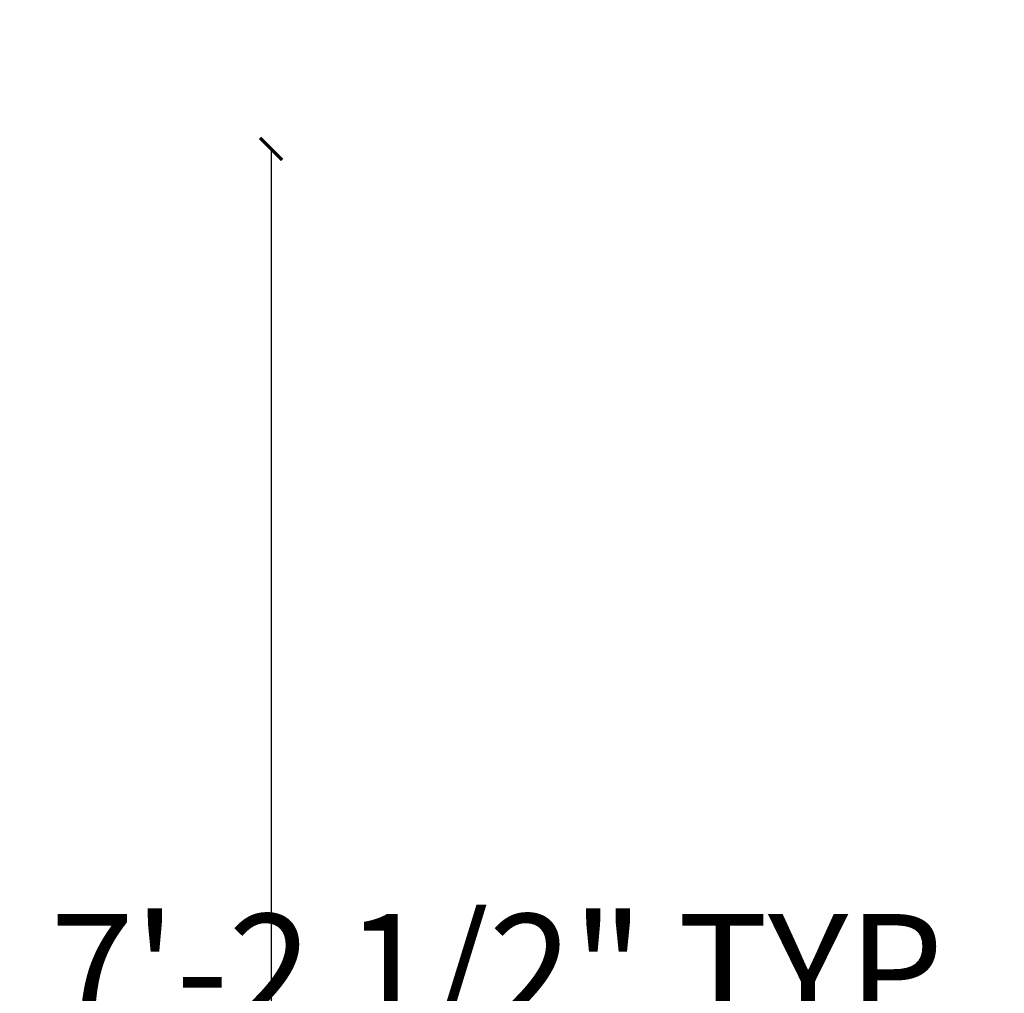
# Model space of a CAD drawing. Units: inches. Extents: x 1858 to 2399, y 1317 to 1943.
# Tile 8 of 8: x 2288 to 2399, y 1742 to 1852. Entities that reach past the tile are written whole.
import ezdxf

# ---------------------------------------------------------------- set-up
doc = ezdxf.new("R2010")
doc.units = ezdxf.units.IN
doc.layers.add('A-ANNO-DIMS', color=2, linetype='Continuous', lineweight=18)
doc.styles.get("Standard").update_dxf_attribs({"font": 'arial.ttf'})
doc.dimstyles.new('ISO-25', dxfattribs={"dimtxt": 12.5, "dimasz": 2.5, "dimexe": 1.25, "dimexo": 0.625, "dimtad": 1, "dimdec": 0, "dimlunit": 4, "dimtxsty": 'Standard', "dimblk": 'ARCHTICK', "dimcen": 2.5, "dimse1": 1, "dimse2": 1, "dimclrd": 3, "dimclrt": 4, "dimadec": 0, "dimazin": 0, "dimtfac": 1, "dimtdec": 0, "dimtmove": 0, "dimatfit": 3, "dimfxl": 1, "dimarcsym": 0})

# ---------------------------------------------------------------- blocks, each defined once
blk = doc.blocks.new('_ArchTick')
at = {"color": 0, "linetype": 'ByBlock', "const_width": 0.15}
blk.add_lwpolyline([(-0.5, -0.5), (0.5, 0.5)], dxfattribs=at)
blk = doc.blocks.new('*D13')
at = {"layer": 'A-ANNO-DIMS', "color": 0, "lineweight": -2, "transparency": 16777216}
blk.add_line((2316.13, 1837.34), (2316.13, 1357.34), dxfattribs=at)
at = {"layer": 'Defpoints', "color": 0, "transparency": 16777216}
for p in [(2273.38, 1837.34), (2273.38, 1357.34), (2316.13, 1357.34)]:
    blk.add_point(p, dxfattribs=at)
at = {"layer": 'A-ANNO-DIMS', "color": 0, "lineweight": -2, "transparency": 16777216, "xscale": 2.5, "yscale": 2.5, "zscale": 2.5}
for p, rotation in [((2316.13, 1837.34), 90), ((2316.13, 1357.34), 270)]:
    blk.add_blockref('_ArchTick', p, dxfattribs=dict(at, rotation=rotation))
at = {"layer": 'A-ANNO-DIMS', "color": 0, "transparency": 16777216, "insert": (2309.12, 1597.34), "char_height": 12.5, "attachment_point": 5, "rotation": 90}
blk.add_mtext("40'", dxfattribs=at)
blk = doc.blocks.new('*D15')
at = {"layer": 'A-ANNO-DIMS', "color": 3, "lineweight": -2, "transparency": 16777216}
for p, q in [((2163.42, 1735.85), (2249.76, 1735.85)), ((2249.76, 1735.85), (2399.03, 1735.85))]:
    blk.add_line(p, q, dxfattribs=at)
at = {"layer": 'Defpoints', "color": 0, "transparency": 16777216}
for p in [(2163.42, 1748.8), (2249.76, 1748.8), (2249.76, 1735.85)]:
    blk.add_point(p, dxfattribs=at)
at = {"layer": 'A-ANNO-DIMS', "color": 3, "lineweight": -2, "transparency": 16777216, "xscale": 2.5, "yscale": 2.5, "zscale": 2.5, "rotation": 180}
blk.add_blockref('_ArchTick', (2163.42, 1735.85), dxfattribs=at)
at = {"layer": 'A-ANNO-DIMS', "color": 3, "lineweight": -2, "transparency": 16777216, "xscale": 2.5, "yscale": 2.5, "zscale": 2.5}
blk.add_blockref('_ArchTick', (2249.76, 1735.85), dxfattribs=at)
at = {"layer": 'A-ANNO-DIMS', "color": 4, "transparency": 16777216, "insert": (2325.64, 1742.94), "char_height": 12.5, "attachment_point": 5}
blk.add_mtext('BED 7\'-2 1/2" TYP.', dxfattribs=at)
blk = doc.blocks.new('*D17')
at = {"layer": 'A-ANNO-DIMS', "color": 3, "lineweight": -2, "transparency": 16777216}
for p, q in [((2276.18, 1653.07), (2276.18, 1851.95)), ((2276.18, 1574.39), (2276.18, 1653.07))]:
    blk.add_line(p, q, dxfattribs=at)
at = {"layer": 'Defpoints', "color": 0, "transparency": 16777216}
for p in [(2264.38, 1653.07), (2276.18, 1653.07), (2264.38, 1574.39)]:
    blk.add_point(p, dxfattribs=at)
at = {"layer": 'A-ANNO-DIMS', "color": 3, "lineweight": -2, "transparency": 16777216, "xscale": 2.5, "yscale": 2.5, "zscale": 2.5}
for p, rotation in [((2276.18, 1653.07), 90), ((2276.18, 1574.39), 270)]:
    blk.add_blockref('_ArchTick', p, dxfattribs=dict(at, rotation=rotation))
at = {"layer": 'A-ANNO-DIMS', "color": 4, "transparency": 16777216, "insert": (2269.09, 1753.76), "char_height": 12.5, "attachment_point": 5, "rotation": 90}
blk.add_mtext('CORNER SOFA 6\'-6 1/2"', dxfattribs=at)

msp = doc.modelspace()

# ---------------------------------------------------------------- dimensions: what is measured, and where the dimension line sits
at = {"layer": 'A-ANNO-DIMS'}
dim = msp.add_linear_dim(base=(2276.18, 1653.07), p1=(2264.38, 1574.39), p2=(2264.38, 1653.07), angle=90, text='CORNER SOFA <>', dimstyle='ISO-25', override={"dimdec": 1, "dimlfac": 1, "dimrnd": 0, "dimzin": 1, "dimdsep": 46, "dimlunit": 4, "dimfrac": 2}, dxfattribs=at)
dim.commit()
dim.dimension.update_dxf_attribs({"geometry": '*D17', "text_midpoint": (2269.09, 1753.76)})
dim = msp.add_linear_dim(base=(2316.13, 1357.34), p1=(2273.38, 1837.34), p2=(2273.38, 1357.34), angle=90, dimstyle='ISO-25', override={"dimclrd": 0, "dimclre": 0, "dimclrt": 0}, dxfattribs=at)
dim.commit()
dim.dimension.update_dxf_attribs({"geometry": '*D13', "text_midpoint": (2309.12, 1597.34)})
dim = msp.add_linear_dim(base=(2249.76, 1735.85), p1=(2163.42, 1748.8), p2=(2249.76, 1748.8), text='BED <> TYP.', dimstyle='ISO-25', override={"dimdec": 1, "dimlfac": 1, "dimrnd": 0, "dimzin": 1, "dimdsep": 46, "dimlunit": 4, "dimfrac": 2}, dxfattribs=at)
dim.commit()
dim.dimension.update_dxf_attribs({"geometry": '*D15', "text_midpoint": (2325.64, 1742.94)})

doc.saveas('drawing.dxf')
